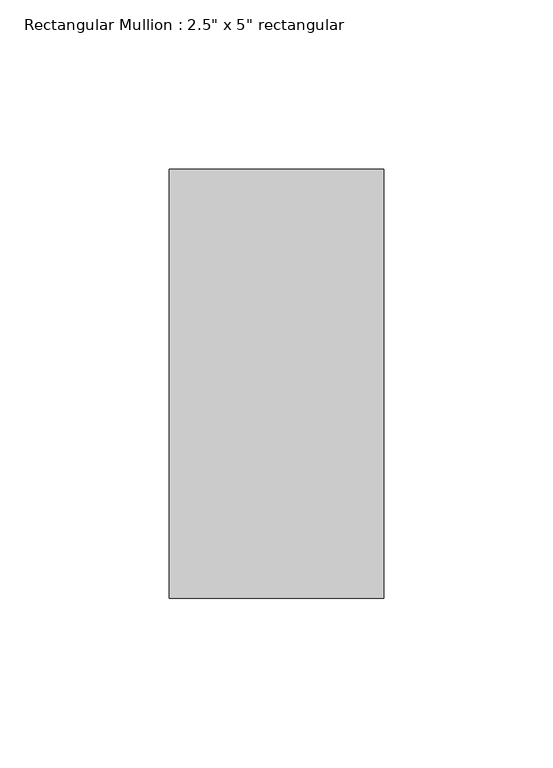
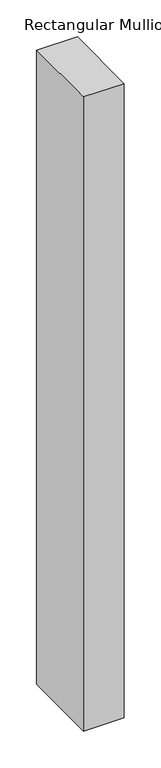
"""IFC4 building model written with IfcOpenShell, lengths in millimetres: member geometry."""

from ifc_helpers import new_model, si_unit, frame, origin, place, context, project, spatial, polyline, outline, extrude, source, transform, mapped, element, save


def member_78934672(model_context):
    return source(origin(), model_context, "Body", "SweptSolid", [
        extrude(outline(polyline([(0.0, 63.5), (0.0, -63.5), (-63.5, -63.5), (-63.5, 63.5), (0.0, 63.5)])), frame((0.0, 0.0, -1047.75), z_axis=(0.0, 0.0, 1.0), x_axis=(1.0, 0.0, 0.0)), (0.0, 0.0, 1.0), 1047.75),
    ])


if __name__ == "__main__":
    model = new_model("IFC4")
    model_context = context("Model", 3, world=origin())
    ifc_project = project(units=[si_unit("LENGTHUNIT", "METRE", prefix="MILLI")], contexts=[model_context])
    site = spatial("IfcSite", under=ifc_project)
    building = spatial("IfcBuilding", under=site)
    placement = place(None, origin())
    member_shape = member_78934672(model_context)
    element("IfcMember", 1, ObjectType="Rectangular Mullion : 2.5\" x 5\" rectangular", at=placement, inside=building, context=model_context, shape_type="MappedRepresentation", body=[
        mapped(member_shape, transform((0.0, 0.0, 0.0), x_axis=(1.0, 0.0, 0.0), y_axis=(0.0, 1.0, 0.0), z_axis=(0.0, 0.0, 1.0))),
    ])
    save(model, "model.ifc")

# Revit data of these elements
# Type "Rectangular Mullion : 2.5\" x 5\" rectangular"
#   built-in parameter 1007304 = 0.416667 (stored number, unit not read)
#   built-in parameter 1007301 = 0.104167 (stored number, unit not read)
#   built-in parameter 1007300 = 0.104167 (stored number, unit not read)
# Element 1 (IfcMember, "Rectangular Mullion : 2.5\" x 5\" rectangular")
#   Materials on its faces: "Iron, Ductile"
# Materials
#   "Iron, Ductile": class "Metal", colour RGB 0 0 0, transparency 0, Description = "Ductile cast iron", Cost = 0
